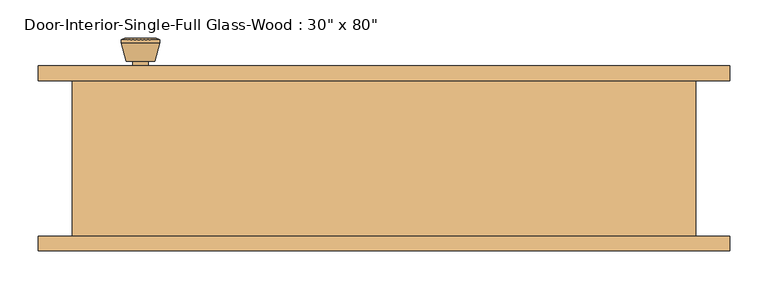
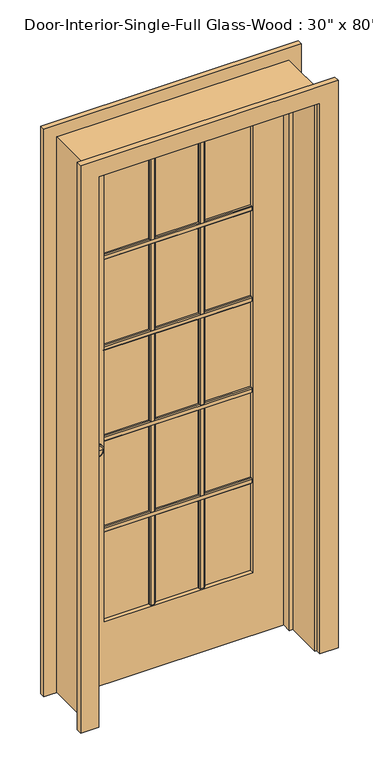
"""IFC4 building model written with IfcOpenShell, lengths in millimetres: door geometry."""

from ifc_helpers import new_model, si_unit, point, frame, frame_2d, origin, place, context, project, spatial, polyline, circle_curve, trimmed, segment, composite_curve, outline, extrude, faceted_brep, source, transform, mapped, element, save
from ifc_brep_helpers import plane_surface, cylinder_surface, revolved_surface, advanced_brep


def door_fe2643c7(model_context):
    return source(origin(), model_context, "Body", "SolidModel", [
        extrude(outline(polyline([(84.455, 1586.23), (90.805, 1586.23), (93.98, 1583.055), (93.98, 1570.355), (90.805, 1567.18), (84.455, 1567.18), (84.455, 1586.23)])), frame((-260.35, 0.0, 0.0), z_axis=(1.0, 0.0, 0.0), x_axis=(0.0, 1.0, 0.0)), (0.0, 0.0, 1.0), 520.7),
        extrude(outline(polyline([(84.455, 1249.9975), (90.805, 1249.9975), (93.98, 1246.8225), (93.98, 1234.1225), (90.805, 1230.9475), (84.455, 1230.9475), (84.455, 1249.9975)])), frame((-260.35, 0.0, 0.0), z_axis=(1.0, 0.0, 0.0), x_axis=(0.0, 1.0, 0.0)), (0.0, 0.0, 1.0), 520.7),
        extrude(outline(polyline([(84.455, 913.765), (90.805, 913.765), (93.98, 910.59), (93.98, 897.89), (90.805, 894.715), (84.455, 894.715), (84.455, 913.765)])), frame((-260.35, 0.0, 0.0), z_axis=(1.0, 0.0, 0.0), x_axis=(0.0, 1.0, 0.0)), (0.0, 0.0, 1.0), 520.7),
        extrude(outline(polyline([(84.455, 577.5325), (90.805, 577.5325), (93.98, 574.3575), (93.98, 561.6575), (90.805, 558.4825), (84.455, 558.4825), (84.455, 577.5325)])), frame((-260.35, 0.0, 0.0), z_axis=(1.0, 0.0, 0.0), x_axis=(0.0, 1.0, 0.0)), (0.0, 0.0, 1.0), 520.7),
        extrude(outline(polyline([(77.2583333, 84.455), (77.2583333, 90.805), (80.4333333, 93.98), (93.1333333, 93.98), (96.3083333, 90.805), (96.3083333, 84.455), (77.2583333, 84.455)])), frame((0.0, 0.0, 231.775), z_axis=(0.0, 0.0, 1.0), x_axis=(1.0, 0.0, 0.0)), (0.0, 0.0, 1.0), 1681.1625),
        extrude(outline(polyline([(-96.3083333, 84.455), (-96.3083333, 90.805), (-93.1333333, 93.98), (-80.4333333, 93.98), (-77.2583333, 90.805), (-77.2583333, 84.455), (-96.3083333, 84.455)])), frame((0.0, 0.0, 231.775), z_axis=(0.0, 0.0, 1.0), x_axis=(1.0, 0.0, 0.0)), (0.0, 0.0, 1.0), 1681.1625),
        extrude(outline(polyline([(77.47, 1586.23), (77.47, 1567.18), (71.12, 1567.18), (67.945, 1570.355), (67.945, 1583.055), (71.12, 1586.23), (77.47, 1586.23)])), frame((-260.35, 0.0, 0.0), z_axis=(1.0, 0.0, 0.0), x_axis=(0.0, 1.0, 0.0)), (0.0, 0.0, 1.0), 520.7),
        extrude(outline(polyline([(77.47, 1249.9975), (77.47, 1230.9475), (71.12, 1230.9475), (67.945, 1234.1225), (67.945, 1246.8225), (71.12, 1249.9975), (77.47, 1249.9975)])), frame((-260.35, 0.0, 0.0), z_axis=(1.0, 0.0, 0.0), x_axis=(0.0, 1.0, 0.0)), (0.0, 0.0, 1.0), 520.7),
        extrude(outline(polyline([(77.47, 913.765), (77.47, 894.715), (71.12, 894.715), (67.945, 897.89), (67.945, 910.59), (71.12, 913.765), (77.47, 913.765)])), frame((-260.35, 0.0, 0.0), z_axis=(1.0, 0.0, 0.0), x_axis=(0.0, 1.0, 0.0)), (0.0, 0.0, 1.0), 520.7),
        extrude(outline(polyline([(77.47, 577.5325), (77.47, 558.4825), (71.12, 558.4825), (67.945, 561.6575), (67.945, 574.3575), (71.12, 577.5325), (77.47, 577.5325)])), frame((-260.35, 0.0, 0.0), z_axis=(1.0, 0.0, 0.0), x_axis=(0.0, 1.0, 0.0)), (0.0, 0.0, 1.0), 520.7),
        extrude(outline(polyline([(77.2583333, 77.47), (96.3083333, 77.47), (96.3083333, 71.12), (93.1333333, 67.945), (80.4333333, 67.945), (77.2583333, 71.12), (77.2583333, 77.47)])), frame((0.0, 0.0, 231.775), z_axis=(0.0, 0.0, 1.0), x_axis=(1.0, 0.0, 0.0)), (0.0, 0.0, 1.0), 1681.1625),
        extrude(outline(polyline([(-96.3083333, 77.47), (-77.2583333, 77.47), (-77.2583333, 71.12), (-80.4333333, 67.945), (-93.1333333, 67.945), (-96.3083333, 71.12), (-96.3083333, 77.47)])), frame((0.0, 0.0, 231.775), z_axis=(0.0, 0.0, 1.0), x_axis=(1.0, 0.0, 0.0)), (0.0, 0.0, 1.0), 1681.1625),
        advanced_brep(
        [(-317.5, 57.5, 914.4), (-307.5, 57.5, 914.4), (-327.5, 57.5, 914.4), (-297.0241324, 8.5, 914.4), (-317.5, 8.5, 914.4), (-337.9758676, 8.5, 914.4), (-292.5, 10.3278681, 914.4), (-342.5, 10.3278681, 914.4), (-292.5, 13.7915463, 914.4), (-342.5, 13.7915463, 914.4), (-298.863764, 38.5, 914.4), (-336.136236, 38.5, 914.4), (-307.5, 38.5, 914.4), (-327.5, 38.5, 914.4)],
        [
            (0, 1),
            (1, 2, circle_curve(frame((-317.5, 57.5, 914.4), z_axis=(0.0, 1.0, 0.0), x_axis=(-1.0, 0.0, 0.0)), 10.0)),
            (2, 0),
            (2, 1, circle_curve(frame((-317.5, 57.5, 914.4), z_axis=(0.0, 1.0, 0.0), x_axis=(-1.0, 0.0, 0.0)), 10.0)),
            (3, 4),
            (4, 5),
            (5, 3, circle_curve(frame((-317.5, 8.5, 914.4), z_axis=(0.0, -1.0, 0.0), x_axis=(-1.0, 0.0, 0.0)), 20.4758676)),
            (3, 5, circle_curve(frame((-317.5, 8.5, 914.4), z_axis=(0.0, -1.0, 0.0), x_axis=(-1.0, 0.0, 0.0)), 20.4758676)),
            (6, 3),
            (5, 7),
            (7, 6, circle_curve(frame((-317.5, 10.3278681, 914.4), z_axis=(0.0, -1.0, 0.0), x_axis=(-1.0, 0.0, 0.0)), 25.0)),
            (6, 7, circle_curve(frame((-317.5, 10.3278681, 914.4), z_axis=(0.0, -1.0, 0.0), x_axis=(-1.0, 0.0, 0.0)), 25.0)),
            (8, 6),
            (7, 9),
            (9, 8, circle_curve(frame((-317.5, 13.7915463, 914.4), z_axis=(0.0, -1.0, 0.0), x_axis=(-1.0, 0.0, 0.0)), 25.0)),
            (8, 9, circle_curve(frame((-317.5, 13.7915463, 914.4), z_axis=(0.0, -1.0, 0.0), x_axis=(-1.0, 0.0, 0.0)), 25.0)),
            (10, 8),
            (9, 11),
            (11, 10, circle_curve(frame((-317.5, 38.5, 914.4), z_axis=(0.0, -1.0, 0.0), x_axis=(-1.0, 0.0, 0.0)), 18.636236)),
            (10, 11, circle_curve(frame((-317.5, 38.5, 914.4), z_axis=(0.0, -1.0, 0.0), x_axis=(-1.0, 0.0, 0.0)), 18.636236)),
            (12, 10),
            (11, 13),
            (13, 12, circle_curve(frame((-317.5, 38.5, 914.4), z_axis=(0.0, -1.0, 0.0), x_axis=(-1.0, 0.0, 0.0)), 10.0)),
            (12, 13, circle_curve(frame((-317.5, 38.5, 914.4), z_axis=(0.0, -1.0, 0.0), x_axis=(-1.0, 0.0, 0.0)), 10.0)),
            (1, 12),
            (13, 2),
        ],
        [
            plane_surface(frame((-317.5, 57.5, 914.4), z_axis=(0.0, 1.0, 0.0), x_axis=(-1.0, 0.0, 0.0))),
            plane_surface(frame((-317.5, 8.5, 914.4), z_axis=(0.0, -1.0, 0.0), x_axis=(-1.0, 0.0, 0.0))),
            revolved_surface(polyline([(-337.9758676, 8.5, 914.4), (-342.5, 10.3278681, 914.4)]), (-317.5, 57.5, 914.4), (0.0, 1.0, 0.0)),
            cylinder_surface(frame((-317.5, 57.5, 914.4), z_axis=(0.0, 1.0, 0.0), x_axis=(-1.0, 0.0, 0.0)), 25.0),
            revolved_surface(polyline([(-342.5, 13.7915463, 914.4), (-336.136236, 38.5, 914.4)]), (-317.5, 57.5, 914.4), (0.0, 1.0, 0.0)),
            plane_surface(frame((-317.5, 38.5, 914.4), z_axis=(0.0, 1.0, 0.0), x_axis=(-1.0, 0.0, 0.0))),
            cylinder_surface(frame((-317.5, 57.5, 914.4), z_axis=(0.0, 1.0, 0.0), x_axis=(-1.0, 0.0, 0.0)), 10.0),
        ],
        [
            (0, [[1, 2, 3]]),
            (0, [[-3, 4, -1]]),
            (1, [[5, 6, 7]]),
            (1, [[-6, -5, 8]]),
            (2, [[9, -7, 10, 11]]),
            (2, [[-10, -8, -9, 12]]),
            (3, [[13, -11, 14, 15]]),
            (3, [[-14, -12, -13, 16]]),
            (4, [[17, -15, 18, 19]]),
            (4, [[-18, -16, -17, 20]]),
            (5, [[21, -19, 22, 23]]),
            (5, [[-22, -20, -21, 24]]),
            (6, [[25, -23, 26, -2]]),
            (6, [[-26, -24, -25, -4]]),
        ],
    ),
        extrude(outline(composite_curve([segment(trimmed(circle_curve(frame_2d((914.4, -317.5)), 30.0), [point((914.4, -347.5))], [point((914.4, -287.5))], False, "CARTESIAN"), True, "CONTINUOUS"), segment(trimmed(circle_curve(frame_2d((914.4, -317.5)), 30.0), [point((914.4, -287.5))], [point((914.4, -347.5))], False, "CARTESIAN"), True, "CONTINUOUS")], self_intersect=False)), frame((0.0, 57.5, 0.0), z_axis=(0.0, 1.0, 0.0), x_axis=(0.0, 0.0, 1.0)), (0.0, 0.0, 1.0), 6.0),
        advanced_brep(
        [(-317.5, 104.425, 914.4), (-327.5, 104.425, 914.4), (-307.5, 104.425, 914.4), (-297.0241324, 153.425, 914.4), (-337.9758676, 153.425, 914.4), (-317.5, 153.425, 914.4), (-292.5, 151.5971319, 914.4), (-342.5, 151.5971319, 914.4), (-292.5, 148.1334537, 914.4), (-342.5, 148.1334537, 914.4), (-298.863764, 123.425, 914.4), (-336.136236, 123.425, 914.4), (-307.5, 123.425, 914.4), (-327.5, 123.425, 914.4)],
        [
            (0, 1),
            (1, 2, circle_curve(frame((-317.5, 104.425, 914.4), z_axis=(0.0, -1.0, 0.0), x_axis=(-1.0, 0.0, 0.0)), 10.0)),
            (2, 0),
            (2, 1, circle_curve(frame((-317.5, 104.425, 914.4), z_axis=(0.0, -1.0, 0.0), x_axis=(-1.0, 0.0, 0.0)), 10.0)),
            (3, 4, circle_curve(frame((-317.5, 153.425, 914.4), z_axis=(0.0, 1.0, 0.0), x_axis=(-1.0, 0.0, 0.0)), 20.4758676)),
            (4, 5),
            (5, 3),
            (4, 3, circle_curve(frame((-317.5, 153.425, 914.4), z_axis=(0.0, 1.0, 0.0), x_axis=(-1.0, 0.0, 0.0)), 20.4758676)),
            (6, 7, circle_curve(frame((-317.5, 151.5971319, 914.4), z_axis=(0.0, 1.0, 0.0), x_axis=(-1.0, 0.0, 0.0)), 25.0)),
            (7, 4),
            (3, 6),
            (7, 6, circle_curve(frame((-317.5, 151.5971319, 914.4), z_axis=(0.0, 1.0, 0.0), x_axis=(-1.0, 0.0, 0.0)), 25.0)),
            (8, 9, circle_curve(frame((-317.5, 148.1334537, 914.4), z_axis=(0.0, 1.0, 0.0), x_axis=(-1.0, 0.0, 0.0)), 25.0)),
            (9, 7),
            (6, 8),
            (9, 8, circle_curve(frame((-317.5, 148.1334537, 914.4), z_axis=(0.0, 1.0, 0.0), x_axis=(-1.0, 0.0, 0.0)), 25.0)),
            (10, 11, circle_curve(frame((-317.5, 123.425, 914.4), z_axis=(0.0, 1.0, 0.0), x_axis=(-1.0, 0.0, 0.0)), 18.636236)),
            (11, 9),
            (8, 10),
            (11, 10, circle_curve(frame((-317.5, 123.425, 914.4), z_axis=(0.0, 1.0, 0.0), x_axis=(-1.0, 0.0, 0.0)), 18.636236)),
            (12, 13, circle_curve(frame((-317.5, 123.425, 914.4), z_axis=(0.0, 1.0, 0.0), x_axis=(-1.0, 0.0, 0.0)), 10.0)),
            (13, 11),
            (10, 12),
            (13, 12, circle_curve(frame((-317.5, 123.425, 914.4), z_axis=(0.0, 1.0, 0.0), x_axis=(-1.0, 0.0, 0.0)), 10.0)),
            (1, 13),
            (12, 2),
        ],
        [
            plane_surface(frame((-317.5, 104.425, 914.4), z_axis=(0.0, -1.0, 0.0), x_axis=(-1.0, 0.0, 0.0))),
            plane_surface(frame((-317.5, 153.425, 914.4), z_axis=(0.0, 1.0, 0.0), x_axis=(-1.0, 0.0, 0.0))),
            revolved_surface(polyline([(-337.9758676, 153.425, 914.4), (-342.5, 151.5971319, 914.4)]), (-317.5, 104.425, 914.4), (0.0, -1.0, 0.0)),
            cylinder_surface(frame((-317.5, 104.425, 914.4), z_axis=(0.0, -1.0, 0.0), x_axis=(-1.0, 0.0, 0.0)), 25.0),
            revolved_surface(polyline([(-342.5, 148.1334537, 914.4), (-336.136236, 123.425, 914.4)]), (-317.5, 104.425, 914.4), (0.0, -1.0, 0.0)),
            plane_surface(frame((-317.5, 123.425, 914.4), z_axis=(0.0, -1.0, 0.0), x_axis=(-1.0, 0.0, 0.0))),
            cylinder_surface(frame((-317.5, 104.425, 914.4), z_axis=(0.0, -1.0, 0.0), x_axis=(-1.0, 0.0, 0.0)), 10.0),
        ],
        [
            (0, [[1, 2, 3]]),
            (0, [[-3, 4, -1]]),
            (1, [[5, 6, 7]]),
            (1, [[8, -7, -6]]),
            (2, [[9, 10, -5, 11]]),
            (2, [[12, -11, -8, -10]]),
            (3, [[13, 14, -9, 15]]),
            (3, [[16, -15, -12, -14]]),
            (4, [[17, 18, -13, 19]]),
            (4, [[20, -19, -16, -18]]),
            (5, [[21, 22, -17, 23]]),
            (5, [[24, -23, -20, -22]]),
            (6, [[-2, 25, -21, 26]]),
            (6, [[-4, -26, -24, -25]]),
        ],
    ),
        extrude(outline(composite_curve([segment(trimmed(circle_curve(frame_2d((914.4, -317.5)), 30.0), [point((914.4, -347.5))], [point((914.4, -287.5))], False, "CARTESIAN"), True, "CONTINUOUS"), segment(trimmed(circle_curve(frame_2d((914.4, -317.5)), 30.0), [point((914.4, -287.5))], [point((914.4, -347.5))], False, "CARTESIAN"), True, "CONTINUOUS")], self_intersect=False)), frame((0.0, 98.425, 0.0), z_axis=(0.0, 1.0, 0.0), x_axis=(0.0, 0.0, 1.0)), (0.0, 0.0, 1.0), 6.0),
        extrude(outline(polyline([(2032.0, -381.0), (0.0, -381.0), (0.0, 381.0), (2032.0, 381.0), (2032.0, -381.0)]), holes=[polyline([(1912.9375, -260.35), (1912.9375, 260.35), (231.775, 260.35), (231.775, -260.35), (1912.9375, -260.35)])]), frame((0.0, 63.5, 0.0), z_axis=(0.0, 1.0, 0.0), x_axis=(0.0, 0.0, 1.0)), (0.0, 0.0, 1.0), 34.925),
        faceted_brep([(406.4, 98.425, 0.0), (406.4, -104.775, 0.0), (381.0, -104.775, 0.0), (381.0, 28.575, 0.0), (368.3, 28.575, 0.0), (368.3, 63.5, 0.0), (381.0, 63.5, 0.0), (381.0, 98.425, 0.0), (406.4, 98.425, 2057.4), (406.4, -104.775, 2057.4), (-406.4, -104.775, 2057.4), (-406.4, -104.775, 0.0), (-381.0, -104.775, 0.0), (-381.0, -104.775, 2032.0), (381.0, -104.775, 2032.0), (381.0, 28.575, 2032.0), (-381.0, 28.575, 2032.0), (-381.0, 28.575, 0.0), (-368.3, 28.575, 0.0), (-368.3, 28.575, 2019.3), (368.3, 28.575, 2019.3), (368.3, 63.5, 2019.3), (-368.3, 63.5, 2019.3), (-368.3, 63.5, 0.0), (-381.0, 63.5, 0.0), (-381.0, 63.5, 2032.0), (381.0, 63.5, 2032.0), (381.0, 98.425, 2032.0), (-381.0, 98.425, 2032.0), (-381.0, 98.425, 0.0), (-406.4, 98.425, 0.0), (-406.4, 98.425, 2057.4)], [[[0, 1, 2, 3, 4, 5, 6, 7]], [[1, 0, 8, 9]], [[2, 1, 9, 10, 11, 12, 13, 14]], [[3, 2, 14, 15]], [[4, 3, 15, 16, 17, 18, 19, 20]], [[5, 4, 20, 21]], [[6, 5, 21, 22, 23, 24, 25, 26]], [[7, 6, 26, 27]], [[0, 7, 27, 28, 29, 30, 31, 8]], [[9, 8, 31, 10]], [[15, 14, 13, 16]], [[21, 20, 19, 22]], [[27, 26, 25, 28]], [[30, 29, 24, 23, 18, 17, 12, 11]], [[10, 31, 30, 11]], [[16, 13, 12, 17]], [[22, 19, 18, 23]], [[28, 25, 24, 29]]]),
        extrude(outline(polyline([(260.35, 77.47), (-260.35, 77.47), (-260.35, 84.455), (260.35, 84.455), (260.35, 77.47)])), frame((0.0, 0.0, 231.775), z_axis=(0.0, 0.0, 1.0), x_axis=(1.0, 0.0, 0.0)), (0.0, 0.0, 1.0), 1681.1625),
        extrude(outline(polyline([(0.0, 387.35), (0.0, 450.85), (2101.85, 450.85), (2101.85, -450.85), (0.0, -450.85), (0.0, -387.35), (2038.35, -387.35), (2038.35, 387.35), (0.0, 387.35)])), frame((0.0, -123.825, 0.0), z_axis=(0.0, 1.0, 0.0), x_axis=(0.0, 0.0, 1.0)), (0.0, 0.0, 1.0), 19.05),
        extrude(outline(polyline([(0.0, 387.35), (0.0, 450.85), (2101.85, 450.85), (2101.85, -450.85), (0.0, -450.85), (0.0, -387.35), (2038.35, -387.35), (2038.35, 387.35), (0.0, 387.35)])), frame((0.0, 98.425, 0.0), z_axis=(0.0, 1.0, 0.0), x_axis=(0.0, 0.0, 1.0)), (0.0, 0.0, 1.0), 19.05),
    ])


if __name__ == "__main__":
    model = new_model("IFC4")
    model_context = context("Model", 3, world=origin())
    ifc_project = project(units=[si_unit("LENGTHUNIT", "METRE", prefix="MILLI")], contexts=[model_context])
    site = spatial("IfcSite", under=ifc_project)
    building = spatial("IfcBuilding", under=site)
    placement = place(None, origin())
    door_shape = door_fe2643c7(model_context)
    element("IfcDoor", 1, ObjectType="Door-Interior-Single-Full Glass-Wood : 30\" x 80\"", at=placement, inside=building, context=model_context, shape_type="MappedRepresentation", body=[
        mapped(door_shape, transform((0.0, 0.0, 0.0), x_axis=(1.0, 0.0, 0.0), y_axis=(0.0, 1.0, 0.0), z_axis=(0.0, 0.0, 1.0))),
    ])
    save(model, "model.ifc")

# Revit data of these elements
# Type "Door-Interior-Single-Full Glass-Wood : 30\" x 80\""
#   Type Mark = "11"
#   Assembly Code = "C1020300"
#   Analytic Construction = "Wood frame with single clear glass"
#   Top Rail = 0' - 4 11/16"
#   Thickness = 0' - 1 3/8"
#   Thermal Resistance (R) = 1.0102 (h·ft²·°F)/BTU
#   Swing Angle [instance default] = 90.00°
#   Stiles = 0' - 4 3/4"
#   Rough Width = 2' - 8"
#   Rough Height = 6' - 9"
#   Height = 6' - 8"
#   Width = 2' - 6"
#   Heat Transfer Coefficient (U) = 0.9900 BTU/(h·ft²·°F)
#   Bottom Rail = 0' - 9 1/8"
#   Show Grill [instance default] = yes
#   Trim Material = Cherry
#   Panel Material = Cherry
#   Frame Material = Cherry
#   Door Handle Material = Aluminum
#   Visual Light Transmittance = 0
#   Solar Heat Gain Coefficient = 0
#   Wall Closure = (empty or 0)
#   Function = (empty or 0)
# Element 1 (IfcDoor, "Door-Interior-Single-Full Glass-Wood : 30\" x 80\"")
#   Materials on its faces: "Cherry", "Aluminum", "Glass"
# Materials
#   "Cherry": class "Wood", colour RGB 226 177 128, transparency 0, Description = "Prunus Serotina", Cost = 0
#   "Aluminum": class "Metal", colour RGB 247 247 247, transparency 0, Description = "Aluminum 6061", Cost = 0
#   "Glass": class "Glass", colour RGB 0 128 192, transparency 0.75, Description = "Soda Lime Glass", Cost = 0
